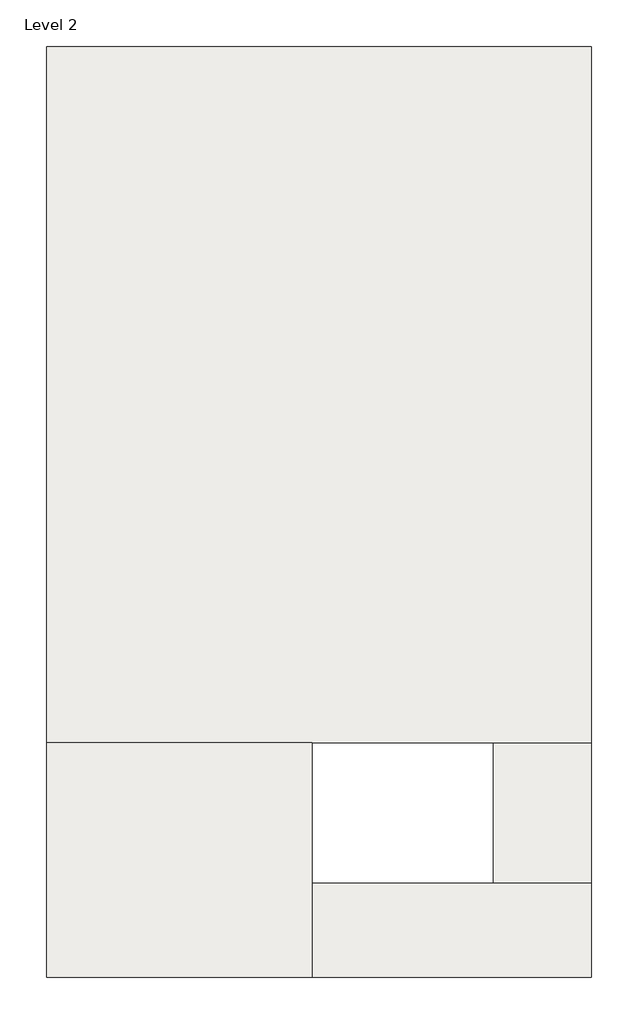
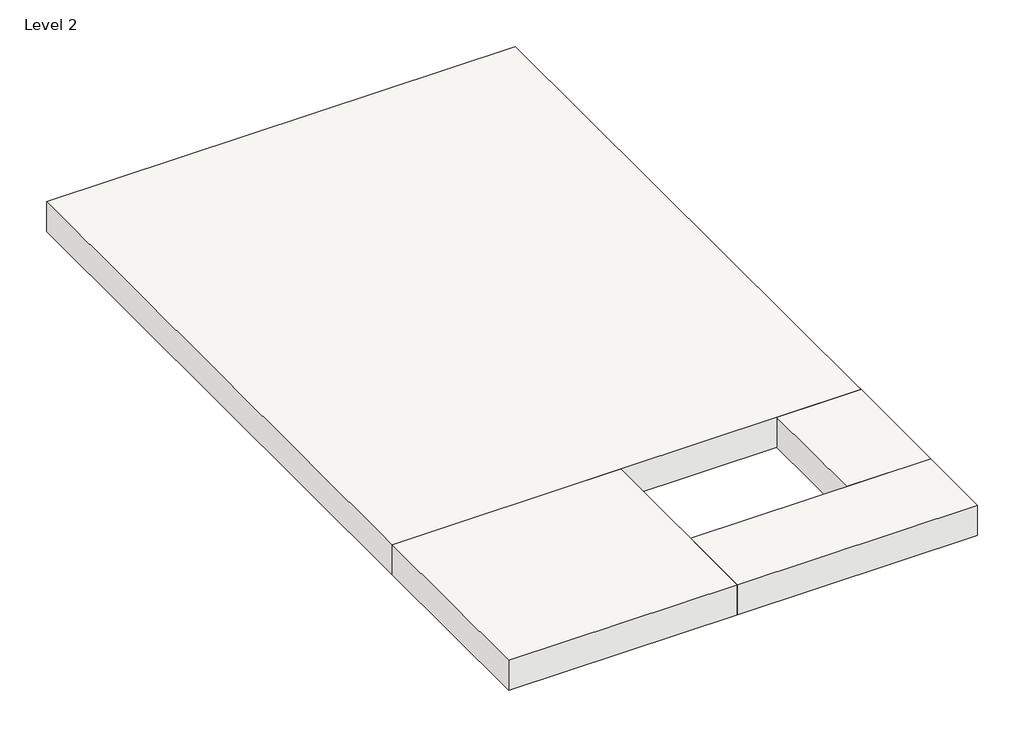
# One storey: 4 roofs.
"""IFC4 building model written with IfcOpenShell, lengths in millimetres."""

from ifc_helpers import new_model, si_unit, frame, origin, place, context, project, spatial, polyline, outline, extrude, element, save

model = new_model("IFC4")

# Units and contexts
model_context = context("Model", 3, world=origin())
ifc_project = project(units=[si_unit("LENGTHUNIT", "METRE", prefix="MILLI")], contexts=[model_context])

# Site, building, storey
site = spatial("IfcSite", under=ifc_project)
building = spatial("IfcBuilding", under=site)
storey = spatial("IfcBuildingStorey", under=building, Name="Level 2", Elevation=3048.0)

# Roofs
placement = place(None, origin())
element("IfcRoof", 1, ObjectType="Steel Truss - Insulation on Metal Deck - EPDM", at=placement, inside=storey, context=model_context, shape_type="SweptSolid", body=[
    extrude(outline(polyline([(-12577.1873398, 11712.5033005), (-4499.9873398, 11712.5033005), (-4499.9873398, 1400.1033005), (-8640.1873398, 1400.1033005), (-12577.1873398, 1400.1033005), (-12577.1873398, 11712.5033005)])), frame((0.0, 0.0, 3048.0), z_axis=(0.0, 0.0, 1.0), x_axis=(1.0, 0.0, 0.0)), (0.0, 0.0, 1.0), 546.1),
])
element("IfcRoof", 2, ObjectType="Steel Truss - Insulation on Metal Deck - EPDM", at=placement, inside=storey, context=model_context, shape_type="SweptSolid", body=[
    extrude(outline(polyline([(-8640.1873398, 1400.1033005), (-8640.1873398, -2079.6966995), (-12577.1873398, -2079.6966995), (-12577.1873398, 1400.1033005), (-8640.1873398, 1400.1033005)])), frame((0.0, 0.0, 3048.0), z_axis=(0.0, 0.0, 1.0), x_axis=(1.0, 0.0, 0.0)), (0.0, 0.0, 1.0), 546.1),
])
element("IfcRoof", 3, ObjectType="Steel Truss - Insulation on Metal Deck - EPDM", at=placement, inside=storey, context=model_context, shape_type="SweptSolid", body=[
    extrude(outline(polyline([(-8640.1873398, -2079.6966995), (-8640.1873398, -885.8966995), (-8640.1873398, -682.6966995), (-4499.9873398, -682.6966995), (-4499.9873398, -2079.6966995), (-8640.1873398, -2079.6966995)])), frame((0.0, 0.0, 3048.0), z_axis=(0.0, 0.0, 1.0), x_axis=(1.0, 0.0, 0.0)), (0.0, 0.0, 1.0), 546.1),
])
element("IfcRoof", 4, ObjectType="Steel Truss - Insulation on Metal Deck - EPDM", at=placement, inside=storey, context=model_context, shape_type="SweptSolid", body=[
    extrude(outline(polyline([(-5947.7873398, -682.6966995), (-5947.7873398, 1425.5033005), (-4499.9873398, 1425.5033005), (-4499.9873398, -682.6966995), (-5947.7873398, -682.6966995)])), frame((0.0, 0.0, 3048.0), z_axis=(0.0, 0.0, 1.0), x_axis=(1.0, 0.0, 0.0)), (0.0, 0.0, 1.0), 546.1),
])

save(model, "model.ifc")

# Revit data of these elements
# Type "Steel Truss - Insulation on Metal Deck - EPDM"
#   Assembly Code = "B1020"
#   Layers, outside or top first: 0' - 0 1/4" "Roofing, EPDM Membrane" (function 4); 0' - 5" "Rigid insulation" (function 3); 0' - 0 1/4" "Metal Deck" (function 1); 1' - 4" "Structure, Steel Bar Joist Layer" (function 1)
# Elements 1, 2, 3, 4 (IfcRoof, "Steel Truss - Insulation on Metal Deck - EPDM")
#   built-in parameter 1001705 = 11.7917 (stored number, unit not read)
#   built-in parameter 1001710 = 33615
#   Phase Created = New Construction
#   Materials on its faces: "Structure, Steel Bar Joist Layer", "Roofing, EPDM Membrane"
# Materials
#   "Roofing, EPDM Membrane": class "Generic", colour RGB 127 127 127, transparency 0, Description = "EPDM roof membrane", Cost = 0
#   "Rigid insulation": class "Generic", colour RGB 127 127 127, transparency 0, Description = "Rigid foam insulation board", Cost = 0
#   "Metal Deck": class "Metal", colour RGB 199 199 199, transparency 0, Description = "Steel, mill finish", Cost = 0
#   "Structure, Steel Bar Joist Layer": class "Metal", colour RGB 127 127 127, transparency 0, Description = "Bar joists, thermal airspace", Cost = 0
